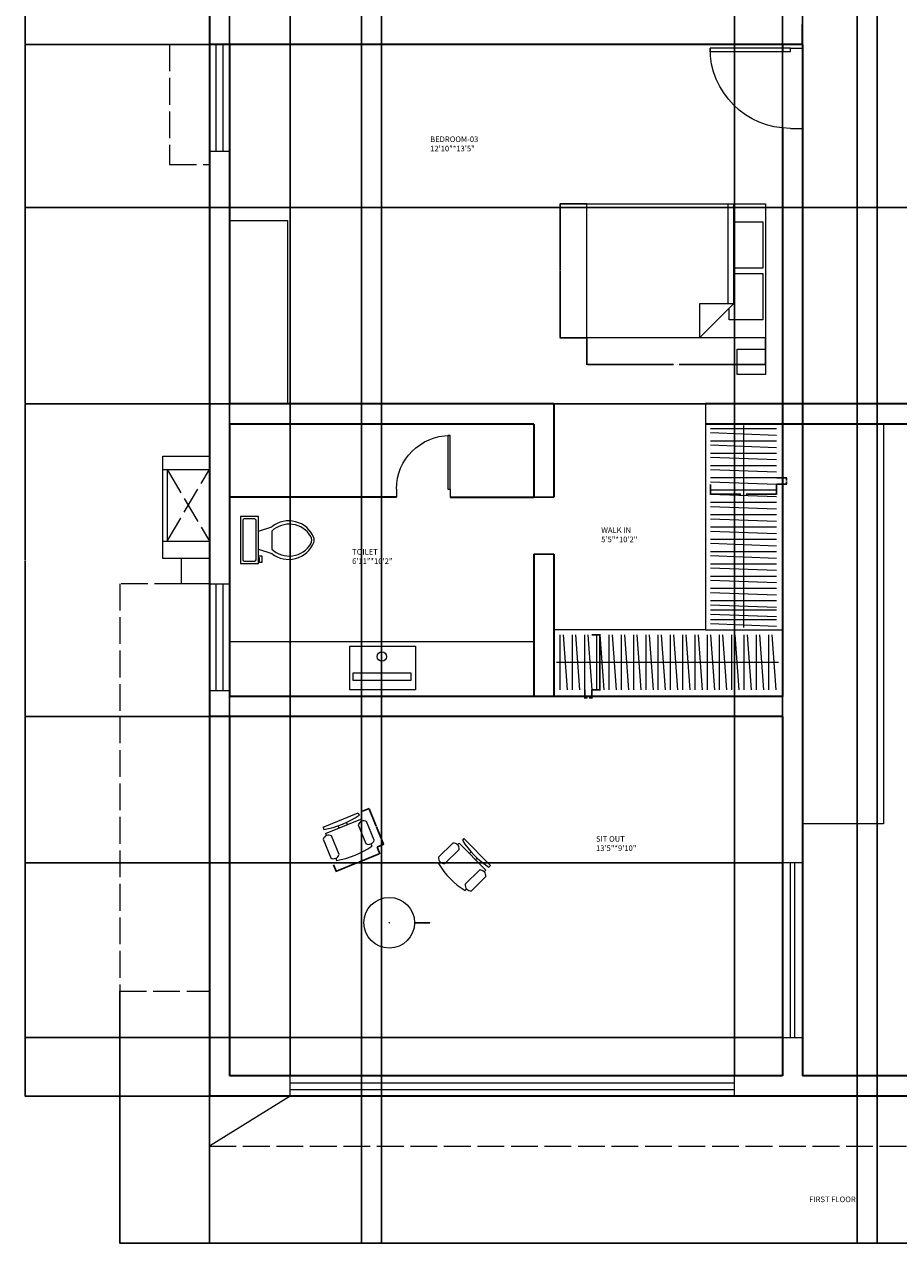
# Model space of a CAD drawing. Units: inches. Extents: x 293720 to 590083, y 155482 to 312405.
# Tile 1 of 4: x 293720 to 294112, y 155482 to 156028. Entities that reach past the tile are written whole.
import ezdxf

# ---------------------------------------------------------------- set-up
doc = ezdxf.new("R2010")
doc.units = ezdxf.units.IN
doc.linetypes.add('ACAD_ISO02W100', pattern=[15, 12, -3])
for name, color, linetype, lineweight in [('A-ANNO-DIMS', 2, 'Continuous', 18), ('A-ANNO-TEXT', 7, 'Continuous', 25), ('A-AREA-IDEN', 7, 'Continuous', 18), ('A-DOOR', 3, 'Continuous', 18), ('A-FLOR-CASE', 8, 'Continuous', 18), ('A-FLOR-FIXT', 9, 'Continuous', 18), ('A-FLOR-OPEN', 8, 'ACAD_ISO02W100', 13), ('A-FLOR-OVHD', 8, 'ACAD_ISO02W100', 13), ('A-FLOR-PROJ', 8, 'Continuous', 18), ('A-FURN', 8, 'Continuous', 18), ('A-GLAZ', 4, 'Continuous', 18), ('A-WALL', 7, 'Continuous', 35), ('A-WALL-HIDN', 7, 'ACAD_ISO02W100', 25)]:
    doc.layers.add(name, color=color, linetype=linetype, lineweight=lineweight)
doc.styles.get("Standard").update_dxf_attribs({"font": 'arial.ttf'})
doc.dimstyles.get("Standard").update_dxf_attribs({"dimtxt": 0.18, "dimasz": 0.18, "dimexe": 0.18, "dimexo": 0.0625, "dimgap": 0.09, "dimtad": 0, "dimtih": 1, "dimtoh": 1, "dimdec": 4, "dimzin": 0, "dimdsep": 46, "dimtxsty": 'Standard', "dimcen": 0.09, "dimadec": 0, "dimazin": 0, "dimtfac": 1, "dimtdec": 4, "dimtofl": 0, "dimtmove": 0, "dimatfit": 3, "dimfxl": 1, "dimtolj": 1, "dimtzin": 0, "dimarcsym": 0})

# ---------------------------------------------------------------- blocks, each defined once
blk = doc.blocks.new('Bed - Queen')
for p, q in [((0, -80.00003), (0, 0)), ((0, 0), (59.99999, 0)), ((59.99999, 0), (59.99999, -80.00003)), ((7.99999, -1.2), (28.79998, -1.2)), ((7.99999, -14.4), (7.99999, -1.2)), ((28.79998, -1.2), (28.79998, -14.4)), ((31.19999, -1.2), (51.99999, -1.2)), ((31.19999, -14.4), (31.19999, -1.2)), ((51.99999, -1.2), (51.99999, -16.4)), ((0, -14.4), (44.8, -14.4)), ((59.99999, -29.6), (44.8, -14.4)), ((44.8, -14.4), (44.8, -29.6)), ((44.8, -16.8), (0, -16.8)), ((51.99999, -16.4), (46.79936, -16.4)), ((44.8, -29.6), (59.99999, -29.6)), ((59.99999, -80.00003), (0, -80.00003))]:
    blk.add_line(p, q)
blk = doc.blocks.new('Toilet - top')
for p, q in [((9.5, -6), (9.5, -2)), ((-10, -8.5), (-8, -8.5)), ((-10, -9.5), (-10, -8.5)), ((-7, -9.5), (-10, -9.5)), ((-8, -8.5), (-8, -8)), ((-7, -8), (-7, -9.5)), ((-4, -8), (-6, -14)), ((4, -8), (6, -14)), ((4, -14), (-4, -14))]:
    blk.add_line(p, q)
blk.add_lwpolyline([(10.5, -8), (10.5, 0), (-10.5, 0), (-10.5, -8)], close=True)
for points in [[(-9.5, -2), (-9.5, -6)], [(8.5, -1), (-8.5, -1)], [(-8.5, -7), (8.5, -7)]]:
    blk.add_lwpolyline(points)
for centre, radius, start, end in [((-8.62, -1.88), 0.884, 81.8699, 188.1301), ((8.62, -1.88), 0.884, 351.8699, 98.1301), ((-8.62, -6.12), 0.884, 171.8699, 278.1301), ((8.62, -6.12), 0.884, 261.8699, 8.1301), ((3.52, -21.58), 12.17, 141.4691, 247.9714), ((4.2, -21.82), 11.33, 136.3677, 238.9468), ((-3.52, -21.58), 12.17, 292.0284, 38.5307), ((-4.2, -21.82), 11.33, 301.053, 43.6321), ((0, -27.88), 4, 245.7318, 294.2682), ((0, -29), 4, 254.8605, 285.1395)]:
    blk.add_arc(centre, radius, start, end)
blk = doc.blocks.new('Chair - Desk')
for p, q in [((-8.5, 0), (-8.5, -1)), ((-8.5, 0), (8.5, 0)), ((8.5, 0), (8.5, -1)), ((-10.5, -5), (-10.5, -14)), ((-8.5, -3), (-8.5, -4)), ((-8.5, -3), (8.5, -3)), ((-6.5, -14), (-6.5, -5)), ((-2, -3), (-2, -1.9355)), ((2, -1.9576), (2, -3)), ((6.5, -5), (6.5, -14)), ((8.5, -3), (8.5, -4)), ((10.5, -14), (10.5, -5)), ((-8.5, -15), (-8.5, -16)), ((8.5, -15), (8.5, -16))]:
    blk.add_line(p, q)
for centre, radius, start, end in [((-8.5, -6.5), 2.5, 36.8699, 143.1301), ((0, 34.625), 36.625, 256.5803, 283.4197), ((8.5, -6.5), 2.5, 36.8699, 143.1301), ((-8.5, -12.5), 2.5, 216.8699, 323.1301), ((0, 19.625), 36.625, 256.5803, 283.4197), ((8.5, -12.5), 2.5, 216.8699, 323.1301)]:
    blk.add_arc(centre, radius, start, end)
blk = doc.blocks.new('*U2')
for p, q in [((0, 0), (0, -6)), ((40, 0), (40, -6))]:
    blk.add_line(p, q)
blk.add_lwpolyline([(0, 0), (0, 40), (1.75, 40), (1.75, 0)], close=True)
blk.add_arc((0, 0), 40, 0, 90)
blk = doc.blocks.new('WIN-48IN')
for p, q in [((0, 9), (48, 9)), ((0, 0), (0, 9)), ((0, 6), (48, 6)), ((48, 9), (48, 0)), ((48, 3), (0, 3)), ((48, 0), (0, 0))]:
    blk.add_line(p, q)
blk = doc.blocks.new('WARDROBE-HANGER-24P54IN')
for p, q in [((0, 0), (0, 24.54)), ((1.33, 24.53), (3.14, 0))]:
    blk.add_line(p, q)
blk = doc.blocks.new('WARDROBE-HANGER-29P64IN')
for p, q in [((0, 2.95), (29.64, 2.95)), ((0, 1.08), (29.64, 0))]:
    blk.add_line(p, q)
blk = doc.blocks.new('*D27')
at = {"layer": 'A-ANNO-DIMS', "color": 0, "lineweight": -2, "transparency": 16777216}
for p, q in [((293974.3, 155754.46), (293978.1, 155754.46)), ((293977.92, 155754.28), (293977.92, 155742.37)), ((293977.92, 155730.1), (293977.92, 155742.01)), ((293974.3, 155729.92), (293978.1, 155729.92))]:
    blk.add_line(p, q, dxfattribs=at)
at = {"layer": 'A-ANNO-DIMS', "color": 0, "lineweight": 100, "transparency": 16777216}
for points in [[(293977.89, 155754.28), (293977.95, 155754.28), (293977.92, 155754.46)], [(293977.89, 155730.1), (293977.95, 155730.1), (293977.92, 155729.92)]]:
    blk.add_solid(points, dxfattribs=at)
at = {"layer": 'Defpoints', "color": 0, "lineweight": 100, "transparency": 16777216}
for p in [(293974.24, 155754.46), (293977.92, 155754.46), (293974.24, 155729.92)]:
    blk.add_point(p, dxfattribs=at)
at = {"layer": 'A-ANNO-DIMS', "color": 0, "transparency": 16777216, "insert": (293977.92, 155742.19), "char_height": 0.18, "attachment_point": 5}
blk.add_mtext('\\A1;HANGER C 25 TYP.', dxfattribs=at)
blk = doc.blocks.new('*D28')
at = {"layer": 'A-ANNO-DIMS', "color": 0, "lineweight": -2, "transparency": 16777216}
for p, q in [((293971.09, 155729.86), (293971.09, 155726.06)), ((293974.24, 155729.86), (293974.24, 155726.06)), ((293971.27, 155726.24), (293972.21, 155726.24)), ((293974.06, 155726.24), (293973.12, 155726.24))]:
    blk.add_line(p, q, dxfattribs=at)
at = {"layer": 'A-ANNO-DIMS', "color": 0, "lineweight": 100, "transparency": 16777216}
for points in [[(293971.27, 155726.27), (293971.27, 155726.21), (293971.09, 155726.24)], [(293974.06, 155726.27), (293974.06, 155726.21), (293974.24, 155726.24)]]:
    blk.add_solid(points, dxfattribs=at)
at = {"layer": 'Defpoints', "color": 0, "lineweight": 100, "transparency": 16777216}
for p in [(293971.09, 155729.92), (293974.24, 155729.92), (293974.24, 155726.24)]:
    blk.add_point(p, dxfattribs=at)
at = {"layer": 'A-ANNO-DIMS', "color": 0, "transparency": 16777216, "insert": (293972.66, 155726.24), "char_height": 0.18, "attachment_point": 5}
blk.add_mtext('\\A1;3 TYP.', dxfattribs=at)
blk = doc.blocks.new('*D29')
at = {"layer": 'A-ANNO-DIMS', "color": 0, "lineweight": -2, "transparency": 16777216}
for p, q in [((294027.35, 155821.9), (294027.35, 155817.34)), ((294027.53, 155817.52), (294040.95, 155817.52)), ((294056.82, 155817.52), (294043.4, 155817.52)), ((294057, 155821.9), (294057, 155817.34))]:
    blk.add_line(p, q, dxfattribs=at)
at = {"layer": 'A-ANNO-DIMS', "color": 0, "lineweight": 100, "transparency": 16777216}
for points in [[(294027.53, 155817.55), (294027.53, 155817.49), (294027.35, 155817.52)], [(294056.82, 155817.55), (294056.82, 155817.49), (294057, 155817.52)]]:
    blk.add_solid(points, dxfattribs=at)
at = {"layer": 'Defpoints', "color": 0, "lineweight": 100, "transparency": 16777216}
for p in [(294027.35, 155821.96), (294057, 155821.96), (294057, 155817.52)]:
    blk.add_point(p, dxfattribs=at)
at = {"layer": 'A-ANNO-DIMS', "color": 0, "transparency": 16777216, "insert": (294042.18, 155817.52), "char_height": 0.18, "attachment_point": 5}
blk.add_mtext('\\A1;HANGER D 30 TYP.', dxfattribs=at)
blk = doc.blocks.new('*D30')
at = {"layer": 'A-ANNO-DIMS', "color": 0, "lineweight": -2, "transparency": 16777216}
for p, q in [((294057.06, 155824.91), (294061.63, 155824.91)), ((294061.45, 155824.73), (294061.45, 155823.62)), ((294061.45, 155822.14), (294061.45, 155823.26)), ((294057.06, 155821.96), (294061.63, 155821.96))]:
    blk.add_line(p, q, dxfattribs=at)
at = {"layer": 'A-ANNO-DIMS', "color": 0, "lineweight": 100, "transparency": 16777216}
for points in [[(294061.42, 155824.73), (294061.48, 155824.73), (294061.45, 155824.91)], [(294061.42, 155822.14), (294061.48, 155822.14), (294061.45, 155821.96)]]:
    blk.add_solid(points, dxfattribs=at)
at = {"layer": 'Defpoints', "color": 0, "lineweight": 100, "transparency": 16777216}
for p in [(294057, 155824.91), (294061.45, 155824.91), (294057, 155821.96)]:
    blk.add_point(p, dxfattribs=at)
at = {"layer": 'A-ANNO-DIMS', "color": 0, "transparency": 16777216, "insert": (294061.45, 155823.44), "char_height": 0.18, "attachment_point": 5}
blk.add_mtext('\\A1;3 TYP.', dxfattribs=at)
blk = doc.blocks.new('*D41')
at = {"layer": 'A-ANNO-DIMS', "color": 0, "lineweight": -2, "transparency": 16777216}
for p, q in [((293878.12, 155659.4), (293879.36, 155656.38)), ((293879.13, 155656.48), (293870.02, 155652.76)), ((293858.69, 155651.46), (293859.92, 155648.43)), ((293860.02, 155648.67), (293869.13, 155652.39))]:
    blk.add_line(p, q, dxfattribs=at)
at = {"layer": 'A-ANNO-DIMS', "color": 0, "lineweight": 100, "transparency": 16777216}
for points in [[(293879.12, 155656.51), (293879.14, 155656.45), (293879.29, 155656.55)], [(293860.01, 155648.69), (293860.03, 155648.64), (293859.85, 155648.6)]]:
    blk.add_solid(points, dxfattribs=at)
at = {"layer": 'Defpoints', "color": 0, "lineweight": 100, "transparency": 16777216}
for p in [(293878.1, 155659.46), (293879.29, 155656.55), (293858.66, 155651.51)]:
    blk.add_point(p, dxfattribs=at)
at = {"layer": 'A-ANNO-DIMS', "color": 0, "transparency": 16777216, "insert": (293869.57, 155652.57), "char_height": 0.18, "attachment_point": 5}
blk.add_mtext('\\A1;CHAIR 21 TYP.', dxfattribs=at)
blk = doc.blocks.new('*D42')
at = {"layer": 'A-ANNO-DIMS', "color": 0, "lineweight": -2, "transparency": 16777216}
for p, q in [((293871.6, 155675.53), (293874.62, 155676.77)), ((293874.53, 155676.53), (293877.66, 155668.86)), ((293880.95, 155660.82), (293877.81, 155668.49)), ((293878.16, 155659.48), (293881.18, 155660.72))]:
    blk.add_line(p, q, dxfattribs=at)
at = {"layer": 'A-ANNO-DIMS', "color": 0, "lineweight": 100, "transparency": 16777216}
for points in [[(293874.55, 155676.54), (293874.5, 155676.52), (293874.46, 155676.7)], [(293880.98, 155660.83), (293880.92, 155660.81), (293881.02, 155660.65)]]:
    blk.add_solid(points, dxfattribs=at)
at = {"layer": 'Defpoints', "color": 0, "lineweight": 100, "transparency": 16777216}
for p in [(293871.54, 155675.51), (293874.46, 155676.7), (293878.1, 155659.46)]:
    blk.add_point(p, dxfattribs=at)
at = {"layer": 'A-ANNO-DIMS', "color": 0, "transparency": 16777216, "insert": (293877.74, 155668.68), "char_height": 0.18, "attachment_point": 5}
blk.add_mtext('\\A1;17 TYP.', dxfattribs=at)
blk = doc.blocks.new('*D43')
at = {"layer": 'A-ANNO-DIMS', "color": 0, "lineweight": -2, "transparency": 16777216}
for p, q in [((293972.1, 155887.5), (293972.1, 155875.38)), ((294052.1, 155887.5), (294052.1, 155875.38)), ((293972.28, 155875.56), (294010.8, 155875.56)), ((294051.92, 155875.56), (294013.4, 155875.56))]:
    blk.add_line(p, q, dxfattribs=at)
at = {"layer": 'A-ANNO-DIMS', "color": 0, "lineweight": 100, "transparency": 16777216}
for points in [[(293972.28, 155875.59), (293972.28, 155875.53), (293972.1, 155875.56)], [(294051.92, 155875.59), (294051.92, 155875.53), (294052.1, 155875.56)]]:
    blk.add_solid(points, dxfattribs=at)
at = {"layer": 'Defpoints', "color": 0, "lineweight": 100, "transparency": 16777216}
for p in [(293972.1, 155887.56), (294052.1, 155887.56), (294052.1, 155875.56)]:
    blk.add_point(p, dxfattribs=at)
at = {"layer": 'A-ANNO-DIMS', "color": 0, "transparency": 16777216, "insert": (294012.1, 155875.56), "char_height": 0.18, "attachment_point": 5}
blk.add_mtext('\\A1;QUEEN BED 80 TYP.', dxfattribs=at)
blk = doc.blocks.new('*D44')
at = {"layer": 'A-ANNO-DIMS', "color": 0, "lineweight": -2, "transparency": 16777216}
for p, q in [((293972.04, 155947.56), (293959.92, 155947.56)), ((293960.1, 155947.38), (293960.1, 155917.74)), ((293960.1, 155887.74), (293960.1, 155917.38)), ((293972.04, 155887.56), (293959.92, 155887.56))]:
    blk.add_line(p, q, dxfattribs=at)
at = {"layer": 'A-ANNO-DIMS', "color": 0, "lineweight": 100, "transparency": 16777216}
for points in [[(293960.07, 155947.38), (293960.13, 155947.38), (293960.1, 155947.56)], [(293960.07, 155887.74), (293960.13, 155887.74), (293960.1, 155887.56)]]:
    blk.add_solid(points, dxfattribs=at)
at = {"layer": 'Defpoints', "color": 0, "lineweight": 100, "transparency": 16777216}
for p in [(293972.1, 155947.56), (293960.1, 155887.56), (293972.1, 155887.56)]:
    blk.add_point(p, dxfattribs=at)
at = {"layer": 'A-ANNO-DIMS', "color": 0, "transparency": 16777216, "insert": (293960.1, 155917.56), "char_height": 0.18, "attachment_point": 5}
blk.add_mtext('\\A1;60 TYP.', dxfattribs=at)
blk = doc.blocks.new('*D53')
at = {"layer": 'A-ANNO-DIMS', "color": 0, "lineweight": -2, "transparency": 16777216}
for p, q in [((294499.07, 156062.55), (294499.07, 155481.85)), ((293762.89, 155594.88), (293762.89, 155481.85)), ((293763.07, 155482.03), (294130.59, 155482.03)), ((294498.89, 155482.03), (294131.37, 155482.03))]:
    blk.add_line(p, q, dxfattribs=at)
at = {"layer": 'A-ANNO-DIMS', "color": 0, "lineweight": 100, "transparency": 16777216}
for points in [[(293763.07, 155482.06), (293763.07, 155482), (293762.89, 155482.03)], [(294498.89, 155482.06), (294498.89, 155482), (294499.07, 155482.03)]]:
    blk.add_solid(points, dxfattribs=at)
at = {"layer": 'Defpoints', "color": 0, "lineweight": 100, "transparency": 16777216}
for p in [(294499.07, 156062.61), (293762.89, 155594.94), (294499.07, 155482.03)]:
    blk.add_point(p, dxfattribs=at)
at = {"layer": 'A-ANNO-DIMS', "color": 0, "transparency": 16777216, "insert": (294130.98, 155482.03), "char_height": 0.18, "attachment_point": 5}
blk.add_mtext('\\A1;736.2', dxfattribs=at)
blk = doc.blocks.new('*D56')
at = {"layer": 'A-ANNO-DIMS', "color": 0, "lineweight": -2, "transparency": 16777216}
for p, q in [((293803.09, 156304.87), (293803.09, 155481.85)), ((293871.09, 156304.87), (293871.09, 155481.85)), ((293803.27, 155482.03), (293836.87, 155482.03)), ((293870.91, 155482.03), (293837.31, 155482.03))]:
    blk.add_line(p, q, dxfattribs=at)
at = {"layer": 'A-ANNO-DIMS', "color": 0, "lineweight": 100, "transparency": 16777216}
for points in [[(293803.27, 155482.06), (293803.27, 155482), (293803.09, 155482.03)], [(293870.91, 155482.06), (293870.91, 155482), (293871.09, 155482.03)]]:
    blk.add_solid(points, dxfattribs=at)
at = {"layer": 'Defpoints', "color": 0, "lineweight": 100, "transparency": 16777216}
for p in [(293803.09, 156304.93), (293871.09, 156304.93), (293871.09, 155482.03)]:
    blk.add_point(p, dxfattribs=at)
at = {"layer": 'A-ANNO-DIMS', "color": 0, "transparency": 16777216, "insert": (293837.09, 155482.03), "char_height": 0.18, "attachment_point": 5}
blk.add_mtext('\\A1;68', dxfattribs=at)
blk = doc.blocks.new('*D57')
at = {"layer": 'A-ANNO-DIMS', "color": 0, "lineweight": -2, "transparency": 16777216}
for p, q in [((293880.093104, 156304.865707), (293880.093104, 155481.8534)), ((294093.093104, 156304.865707), (294093.093104, 155481.8534)), ((293880.273104, 155482.0334), (293986.302722, 155482.0334)), ((294092.913104, 155482.0334), (293986.883486, 155482.0334))]:
    blk.add_line(p, q, dxfattribs=at)
at = {"layer": 'A-ANNO-DIMS', "color": 0, "lineweight": 100, "transparency": 16777216}
for points in [[(293880.273104, 155482.0634), (293880.273104, 155482.0034), (293880.093104, 155482.0334)], [(294092.913104, 155482.0634), (294092.913104, 155482.0034), (294093.093104, 155482.0334)]]:
    blk.add_solid(points, dxfattribs=at)
at = {"layer": 'Defpoints', "color": 0, "lineweight": 100, "transparency": 16777216}
for p in [(293880.093104, 156304.928207), (294093.093104, 156304.928207), (294093.093104, 155482.0334)]:
    blk.add_point(p, dxfattribs=at)
at = {"layer": 'A-ANNO-DIMS', "color": 0, "transparency": 16777216, "insert": (293986.593104, 155482.0334), "char_height": 0.18, "attachment_point": 5}
blk.add_mtext('\\A1;213', dxfattribs=at)
blk = doc.blocks.new('*D58')
at = {"layer": 'A-ANNO-DIMS', "color": 0, "lineweight": -2, "transparency": 16777216}
for p, q in [((294102.09, 156200.87), (294102.09, 155481.85)), ((294173.09, 156200.87), (294173.09, 155481.85)), ((294102.27, 155482.03), (294137.39, 155482.03)), ((294172.91, 155482.03), (294137.79, 155482.03))]:
    blk.add_line(p, q, dxfattribs=at)
at = {"layer": 'A-ANNO-DIMS', "color": 0, "lineweight": 100, "transparency": 16777216}
for points in [[(294102.27, 155482.06), (294102.27, 155482), (294102.09, 155482.03)], [(294172.91, 155482.06), (294172.91, 155482), (294173.09, 155482.03)]]:
    blk.add_solid(points, dxfattribs=at)
at = {"layer": 'Defpoints', "color": 0, "lineweight": 100, "transparency": 16777216}
for p in [(294102.09, 156200.93), (294173.09, 156200.93), (294173.09, 155482.03)]:
    blk.add_point(p, dxfattribs=at)
at = {"layer": 'A-ANNO-DIMS', "color": 0, "transparency": 16777216, "insert": (294137.59, 155482.03), "char_height": 0.18, "attachment_point": 5}
blk.add_mtext('\\A1;71', dxfattribs=at)
blk = doc.blocks.new('*D61')
at = {"layer": 'A-ANNO-DIMS', "color": 0, "lineweight": -2, "transparency": 16777216}
for p, q in [((293803.03, 155717.93), (293720.36, 155717.93)), ((293720.54, 155717.75), (293720.54, 155633.11)), ((293720.54, 155548.11), (293720.54, 155632.75)), ((293803.03, 155547.93), (293720.36, 155547.93))]:
    blk.add_line(p, q, dxfattribs=at)
at = {"layer": 'A-ANNO-DIMS', "color": 0, "lineweight": 100, "transparency": 16777216}
for points in [[(293720.51, 155717.75), (293720.57, 155717.75), (293720.54, 155717.93)], [(293720.51, 155548.11), (293720.57, 155548.11), (293720.54, 155547.93)]]:
    blk.add_solid(points, dxfattribs=at)
at = {"layer": 'Defpoints', "color": 0, "lineweight": 100, "transparency": 16777216}
for p in [(293720.54, 155717.93), (293803.09, 155717.93), (293803.09, 155547.93)]:
    blk.add_point(p, dxfattribs=at)
at = {"layer": 'A-ANNO-DIMS', "color": 0, "transparency": 16777216, "insert": (293720.54, 155632.93), "char_height": 0.18, "attachment_point": 5}
blk.add_mtext('\\A1;170', dxfattribs=at)
blk = doc.blocks.new('*D62')
at = {"layer": 'A-ANNO-DIMS', "color": 0, "lineweight": -2, "transparency": 16777216}
for p, q in [((293812.03, 155857.93), (293720.36, 155857.93)), ((293720.54, 155857.75), (293720.54, 155788.11)), ((293720.54, 155718.11), (293720.54, 155787.75)), ((293803.03, 155717.93), (293720.36, 155717.93))]:
    blk.add_line(p, q, dxfattribs=at)
at = {"layer": 'A-ANNO-DIMS', "color": 0, "lineweight": 100, "transparency": 16777216}
for points in [[(293720.51, 155857.75), (293720.57, 155857.75), (293720.54, 155857.93)], [(293720.51, 155718.11), (293720.57, 155718.11), (293720.54, 155717.93)]]:
    blk.add_solid(points, dxfattribs=at)
at = {"layer": 'Defpoints', "color": 0, "lineweight": 100, "transparency": 16777216}
for p in [(293720.54, 155857.93), (293812.09, 155857.93), (293803.09, 155717.93)]:
    blk.add_point(p, dxfattribs=at)
at = {"layer": 'A-ANNO-DIMS', "color": 0, "transparency": 16777216, "insert": (293720.54, 155787.93), "char_height": 0.18, "attachment_point": 5}
blk.add_mtext('\\A1;140', dxfattribs=at)
blk = doc.blocks.new('*D63')
at = {"layer": 'A-ANNO-DIMS', "color": 0, "lineweight": -2, "transparency": 16777216}
for p, q in [((293812.03, 156018.93), (293720.36, 156018.93)), ((293720.54, 156018.75), (293720.54, 155938.61)), ((293720.54, 155858.11), (293720.54, 155938.25)), ((293812.03, 155857.93), (293720.36, 155857.93))]:
    blk.add_line(p, q, dxfattribs=at)
at = {"layer": 'A-ANNO-DIMS', "color": 0, "lineweight": 100, "transparency": 16777216}
for points in [[(293720.51, 156018.75), (293720.57, 156018.75), (293720.54, 156018.93)], [(293720.51, 155858.11), (293720.57, 155858.11), (293720.54, 155857.93)]]:
    blk.add_solid(points, dxfattribs=at)
at = {"layer": 'Defpoints', "color": 0, "lineweight": 100, "transparency": 16777216}
for p in [(293720.54, 156018.93), (293812.09, 156018.93), (293812.09, 155857.93)]:
    blk.add_point(p, dxfattribs=at)
at = {"layer": 'A-ANNO-DIMS', "color": 0, "transparency": 16777216, "insert": (293720.54, 155938.43), "char_height": 0.18, "attachment_point": 5}
blk.add_mtext('\\A1;161', dxfattribs=at)
blk = doc.blocks.new('*D64')
at = {"layer": 'A-ANNO-DIMS', "color": 0, "lineweight": -2, "transparency": 16777216}
for p, q in [((293803.03, 156166.43), (293720.36, 156166.43)), ((293720.54, 156166.25), (293720.54, 156092.86)), ((293720.54, 156019.11), (293720.54, 156092.5)), ((293812.03, 156018.93), (293720.36, 156018.93))]:
    blk.add_line(p, q, dxfattribs=at)
at = {"layer": 'A-ANNO-DIMS', "color": 0, "lineweight": 100, "transparency": 16777216}
for points in [[(293720.51, 156166.25), (293720.57, 156166.25), (293720.54, 156166.43)], [(293720.51, 156019.11), (293720.57, 156019.11), (293720.54, 156018.93)]]:
    blk.add_solid(points, dxfattribs=at)
at = {"layer": 'Defpoints', "color": 0, "lineweight": 100, "transparency": 16777216}
for p in [(293720.54, 156166.43), (293803.09, 156166.43), (293812.09, 156018.93)]:
    blk.add_point(p, dxfattribs=at)
at = {"layer": 'A-ANNO-DIMS', "color": 0, "transparency": 16777216, "insert": (293720.54, 156092.68), "char_height": 0.18, "attachment_point": 5}
blk.add_mtext('\\A1;147.5', dxfattribs=at)
blk = doc.blocks.new('*D66')
at = {"layer": 'A-ANNO-DIMS', "color": 0, "lineweight": -2, "transparency": 16777216}
for p, q in [((293812.09, 155556.99), (293812.09, 156377.57)), ((293812.27, 156377.39), (293825.26, 156377.39)), ((293839.03, 156377.39), (293826.05, 156377.39)), ((293839.21, 155556.99), (293839.21, 156377.57))]:
    blk.add_line(p, q, dxfattribs=at)
at = {"layer": 'A-ANNO-DIMS', "color": 0, "lineweight": 100, "transparency": 16777216}
for points in [[(293812.27, 156377.42), (293812.27, 156377.36), (293812.09, 156377.39)], [(293839.03, 156377.42), (293839.03, 156377.36), (293839.21, 156377.39)]]:
    blk.add_solid(points, dxfattribs=at)
at = {"layer": 'Defpoints', "color": 0, "lineweight": 100, "transparency": 16777216}
for p in [(293839.21, 156377.39), (293812.09, 155556.93), (293839.21, 155556.93)]:
    blk.add_point(p, dxfattribs=at)
at = {"layer": 'A-ANNO-DIMS', "color": 0, "transparency": 16777216, "insert": (293825.65, 156377.39), "char_height": 0.18, "attachment_point": 5}
blk.add_mtext('\\A1;27.12', dxfattribs=at)
blk = doc.blocks.new('*D67')
at = {"layer": 'A-ANNO-DIMS', "color": 0, "lineweight": -2, "transparency": 16777216}
for p, q in [((293839.21, 155556.99), (293839.21, 156377.57)), ((293839.39, 156377.39), (293938.24, 156377.39)), ((294038, 156377.39), (293939.15, 156377.39)), ((294038.18, 155556.99), (294038.18, 156377.57))]:
    blk.add_line(p, q, dxfattribs=at)
at = {"layer": 'A-ANNO-DIMS', "color": 0, "lineweight": 100, "transparency": 16777216}
for points in [[(293839.39, 156377.42), (293839.39, 156377.36), (293839.21, 156377.39)], [(294038, 156377.42), (294038, 156377.36), (294038.18, 156377.39)]]:
    blk.add_solid(points, dxfattribs=at)
at = {"layer": 'Defpoints', "color": 0, "lineweight": 100, "transparency": 16777216}
for p in [(294038.18, 156377.39), (293839.21, 155556.93), (294038.18, 155556.93)]:
    blk.add_point(p, dxfattribs=at)
at = {"layer": 'A-ANNO-DIMS', "color": 0, "transparency": 16777216, "insert": (293938.7, 156377.39), "char_height": 0.18, "attachment_point": 5}
blk.add_mtext('\\A1;198.97', dxfattribs=at)
blk = doc.blocks.new('*D68')
at = {"layer": 'A-ANNO-DIMS', "color": 0, "lineweight": -2, "transparency": 16777216}
for p, q in [((294038.180795, 155556.990707), (294038.180795, 156377.567612)), ((294038.360795, 156377.387612), (294048.417601, 156377.387612)), ((294059.406085, 156377.387612), (294049.349279, 156377.387612)), ((294059.586085, 155556.990707), (294059.586085, 156377.567612))]:
    blk.add_line(p, q, dxfattribs=at)
at = {"layer": 'A-ANNO-DIMS', "color": 0, "lineweight": 100, "transparency": 16777216}
for points in [[(294038.360795, 156377.417612), (294038.360795, 156377.357612), (294038.180795, 156377.387612)], [(294059.406085, 156377.417612), (294059.406085, 156377.357612), (294059.586085, 156377.387612)]]:
    blk.add_solid(points, dxfattribs=at)
at = {"layer": 'Defpoints', "color": 0, "lineweight": 100, "transparency": 16777216}
for p in [(294059.586085, 156377.387612), (294038.180795, 155556.928207), (294059.586085, 155556.928207)]:
    blk.add_point(p, dxfattribs=at)
at = {"layer": 'A-ANNO-DIMS', "color": 0, "transparency": 16777216, "insert": (294048.88344, 156377.387612), "char_height": 0.18, "attachment_point": 5}
blk.add_mtext('\\A1;21.405', dxfattribs=at)
blk = doc.blocks.new('*D69')
at = {"layer": 'A-ANNO-DIMS', "color": 0, "lineweight": -2, "transparency": 16777216}
for p, q in [((294068.586085, 155556.990707), (294068.586085, 156377.567612)), ((294068.766085, 156377.387612), (294096.611145, 156377.387612)), ((294125.103763, 156377.387612), (294097.258703, 156377.387612)), ((294125.283763, 155556.990707), (294125.283763, 156377.567612))]:
    blk.add_line(p, q, dxfattribs=at)
at = {"layer": 'A-ANNO-DIMS', "color": 0, "lineweight": 100, "transparency": 16777216}
for points in [[(294068.766085, 156377.417612), (294068.766085, 156377.357612), (294068.586085, 156377.387612)], [(294125.103763, 156377.417612), (294125.103763, 156377.357612), (294125.283763, 156377.387612)]]:
    blk.add_solid(points, dxfattribs=at)
at = {"layer": 'Defpoints', "color": 0, "lineweight": 100, "transparency": 16777216}
for p in [(294125.283763, 156377.387612), (294068.586085, 155556.928207), (294125.283763, 155556.928207)]:
    blk.add_point(p, dxfattribs=at)
at = {"layer": 'A-ANNO-DIMS', "color": 0, "transparency": 16777216, "insert": (294096.934924, 156377.387612), "char_height": 0.18, "attachment_point": 5}
blk.add_mtext('\\A1;56.7', dxfattribs=at)
blk = doc.blocks.new('*D72')
at = {"layer": 'A-ANNO-DIMS', "color": 0, "lineweight": -2, "transparency": 16777216}
for p, q in [((294321.18, 155945.93), (293720.36, 155945.93)), ((293720.54, 155945.75), (293720.54, 155902.11)), ((293720.54, 155858.11), (293720.54, 155901.75)), ((294321.18, 155857.93), (293720.36, 155857.93))]:
    blk.add_line(p, q, dxfattribs=at)
at = {"layer": 'A-ANNO-DIMS', "color": 0, "lineweight": 100, "transparency": 16777216}
for points in [[(293720.51, 155945.75), (293720.57, 155945.75), (293720.54, 155945.93)], [(293720.51, 155858.11), (293720.57, 155858.11), (293720.54, 155857.93)]]:
    blk.add_solid(points, dxfattribs=at)
at = {"layer": 'Defpoints', "color": 0, "lineweight": 100, "transparency": 16777216}
for p in [(293720.54, 155945.93), (294321.24, 155945.93), (294321.24, 155857.93)]:
    blk.add_point(p, dxfattribs=at)
at = {"layer": 'A-ANNO-DIMS', "color": 0, "transparency": 16777216, "insert": (293720.54, 155901.93), "char_height": 0.18, "attachment_point": 5}
blk.add_mtext('\\A1;88', dxfattribs=at)
blk = doc.blocks.new('*D75')
at = {"layer": 'A-ANNO-DIMS', "color": 0, "lineweight": -2, "transparency": 16777216}
for p, q in [((294059.52, 155652.4), (293720.36, 155652.4)), ((293720.54, 155652.22), (293720.54, 155613.45)), ((293720.54, 155574.32), (293720.54, 155613.09)), ((294059.52, 155574.14), (293720.36, 155574.14))]:
    blk.add_line(p, q, dxfattribs=at)
at = {"layer": 'A-ANNO-DIMS', "color": 0, "lineweight": 100, "transparency": 16777216}
for points in [[(293720.51, 155652.22), (293720.57, 155652.22), (293720.54, 155652.4)], [(293720.51, 155574.32), (293720.57, 155574.32), (293720.54, 155574.14)]]:
    blk.add_solid(points, dxfattribs=at)
at = {"layer": 'Defpoints', "color": 0, "lineweight": 100, "transparency": 16777216}
for p in [(293720.54, 155652.4), (294059.59, 155652.4), (294059.59, 155574.14)]:
    blk.add_point(p, dxfattribs=at)
at = {"layer": 'A-ANNO-DIMS', "color": 0, "transparency": 16777216, "insert": (293720.54, 155613.27), "char_height": 0.18, "attachment_point": 5}
blk.add_mtext('\\A1;78.26', dxfattribs=at)
blk = doc.blocks.new('*D78')
at = {"layer": 'A-ANNO-DIMS', "color": 0, "lineweight": -2, "transparency": 16777216}
for p, q in [((293883.49, 155625.56), (293883.67, 155625.56)), ((293883.58, 155625.47), (293883.58, 155625.65)), ((293901.74, 155625.56), (293895.11, 155625.56))]:
    blk.add_line(p, q, dxfattribs=at)
at = {"layer": 'A-ANNO-DIMS', "color": 0, "lineweight": 100, "transparency": 16777216}
blk.add_solid([(293895.11, 155625.59), (293895.11, 155625.53), (293894.93, 155625.56)], dxfattribs=at)
at = {"layer": 'Defpoints', "color": 0, "lineweight": 100, "transparency": 16777216}
for p in [(293872.24, 155625.56), (293894.93, 155625.56)]:
    blk.add_point(p, dxfattribs=at)
at = {"layer": 'A-ANNO-DIMS', "color": 0, "transparency": 16777216, "insert": (293902.3, 155625.56), "char_height": 0.18, "attachment_point": 5}
blk.add_mtext('\\A1;∅22.692', dxfattribs=at)

msp = doc.modelspace()

# ---------------------------------------------------------------- linework, layer by layer
at = {"layer": 'A-FLOR-CASE'}
for p, q in [((293812.0931, 155940.1253), (293837.9841, 155940.1253)), ((293837.9841, 155940.1253), (293837.9841, 155857.9282)), ((294025.2305, 155857.9282), (294025.2305, 155756.6999)), ((294042.2003, 155848.2167), (294042.2003, 155764.4281)), ((294104.856, 155848.9282), (294104.856, 155669.844)), ((294042.2003, 155764.4281), (294042.2003, 155757.8352)), ((293812.0931, 155751.5862), (293948.3101, 155751.5862)), ((294025.2305, 155756.6999), (293957.3101, 155756.6999)), ((294025.2305, 155756.6999), (294059.5861, 155756.6999)), ((293958.4339, 155742.2401), (294057.8148, 155742.2401)), ((294104.856, 155669.844), (294068.5861, 155669.844))]:
    msp.add_line(p, q, dxfattribs=at)
at = {"layer": 'A-FLOR-FIXT'}
for p, q in [((293867.4587, 155737.5237), (293893.1801, 155737.5237)), ((293867.4587, 155734.0238), (293867.4587, 155737.5237)), ((293893.1801, 155737.5237), (293893.1801, 155734.0238)), ((293893.1801, 155734.0238), (293867.4587, 155734.0238))]:
    msp.add_line(p, q, dxfattribs=at)
msp.add_lwpolyline([(293865.9092, 155749.3986), (293895.3459, 155749.3986), (293895.3459, 155729.8631), (293865.9092, 155729.8631)], close=True, dxfattribs=at)
msp.add_circle((293880.2971, 155744.78), 2.1189, dxfattribs=at)
at = {"layer": 'A-FLOR-OPEN'}
for p, q in [((293784.2178, 155796.4872), (293803.0931, 155828.5172)), ((293784.2178, 155828.5172), (293803.0931, 155796.4872))]:
    msp.add_line(p, q, dxfattribs=at)
at = {"layer": 'A-FLOR-OVHD'}
for p, q in [((293803.0931, 156018.9282), (293785.2239, 156018.9282)), ((293785.2239, 156018.9282), (293785.2239, 155965.1062)), ((293785.2239, 155965.1062), (293803.0931, 155965.1062)), ((293790.4983, 155777.4328), (293762.8891, 155777.4328)), ((293762.8891, 155777.4328), (293762.8891, 155717.9282)), ((293803.0931, 155717.9282), (293762.8891, 155717.9282)), ((293762.8891, 155717.9282), (293762.8891, 155594.9386)), ((293762.8891, 155594.9386), (293803.0931, 155594.9386)), ((293803.0931, 155525.5662), (294266.2589, 155525.5662))]:
    msp.add_line(p, q, dxfattribs=at)
at = {"layer": 'A-FLOR-PROJ'}
for p, q in [((293782.1825, 155828.5172), (293782.1825, 155834.5389)), ((293782.1825, 155834.5389), (293803.0931, 155834.5389)), ((293782.1825, 155796.4872), (293782.1825, 155828.5172)), ((293782.1825, 155828.5172), (293803.0931, 155828.5172)), ((293784.2178, 155828.5172), (293784.2178, 155796.4872)), ((293782.1825, 155788.7451), (293782.1825, 155796.4872)), ((293782.1825, 155796.4872), (293803.0931, 155796.4872)), ((293803.0931, 155788.7451), (293782.1825, 155788.7451)), ((293790.4983, 155777.4328), (293790.4983, 155788.7451)), ((293803.0931, 155777.4328), (293790.4983, 155777.4328)), ((293839.2106, 155547.9282), (293803.0931, 155525.5662)), ((293803.0931, 155525.5662), (293803.0931, 155547.9282))]:
    msp.add_line(p, q, dxfattribs=at)
at = {"layer": 'A-FURN'}
msp.add_lwpolyline([(294039.2942, 155882.4281), (294052.0946, 155882.4281), (294052.0946, 155871.0591), (294039.2942, 155871.0591)], close=True, dxfattribs=at)
msp.add_circle((293883.5815, 155625.5625), 11.3462, dxfattribs=at)
at = {"layer": 'A-GLAZ'}
for p, q in [((294068.5861, 155652.3986), (294059.5861, 155652.3986)), ((294063.0468, 155652.3537), (294063.0468, 155574.1424)), ((294064.9463, 155652.3986), (294064.9463, 155574.1424)), ((294059.5861, 155574.1424), (294068.5861, 155574.1424)), ((293839.2106, 155547.9282), (293839.2106, 155556.9282)), ((294038.1808, 155547.9282), (294038.1808, 155556.9282)), ((293839.2106, 155553.9282), (294038.1808, 155553.9282)), ((293839.2106, 155550.9282), (294038.1808, 155550.9282))]:
    msp.add_line(p, q, dxfattribs=at)
at = {"layer": 'A-WALL'}
for p, q in [((293803.0931, 156313.9282), (293803.0931, 155547.9282)), ((294068.5861, 156018.9282), (294068.5861, 156027.9282)), ((294068.5861, 156018.9282), (293803.0931, 156018.9282)), ((293812.0931, 156018.9282), (293812.0931, 155857.9282)), ((294059.5861, 156018.9282), (294059.5861, 156015.7616)), ((294068.5861, 156018.9282), (294068.5861, 155556.9282)), ((294059.5861, 155981.517), (294059.5861, 155726.9282)), ((293957.3101, 155857.9282), (293812.0931, 155857.9282)), ((293957.3101, 155857.9282), (293957.3101, 155816.1828)), ((294463.2763, 155857.9282), (294025.2305, 155857.9282)), ((293812.0931, 155848.9282), (293812.0931, 155726.9282)), ((293948.3101, 155848.9282), (293812.0931, 155848.9282)), ((293948.3101, 155848.9282), (293948.3101, 155816.1828)), ((294144.2603, 155848.9282), (294025.2305, 155848.9282)), ((293886.7893, 155816.1828), (293812.0931, 155816.1828)), ((293910.7893, 155816.1828), (293948.3101, 155816.1828)), ((293948.3101, 155790.5985), (293948.3101, 155726.9282)), ((293957.3101, 155790.5985), (293957.3101, 155726.9282)), ((294059.5861, 155726.9282), (293812.0931, 155726.9282)), ((294059.5861, 155717.9282), (293803.0931, 155717.9282)), ((293812.0931, 155717.9282), (293812.0931, 155556.9282)), ((294059.5861, 155717.9282), (294059.5861, 155556.9282)), ((294059.5861, 155556.9282), (293812.0931, 155556.9282)), ((294245.5861, 155556.9282), (294068.5861, 155556.9282)), ((294274.4362, 155547.9282), (293803.0931, 155547.9282))]:
    msp.add_line(p, q, dxfattribs=at)
at = {"layer": 'A-WALL-HIDN'}
for p, q in [((293948.3101, 155816.1828), (293957.3101, 155816.1828)), ((293948.3101, 155790.5985), (293957.3101, 155790.5985))]:
    msp.add_line(p, q, dxfattribs=at)

# ---------------------------------------------------------------- block references
at = {"layer": 'A-DOOR', "xscale": -0.9, "yscale": 0.9, "zscale": 0.9, "rotation": 90}
msp.add_blockref('*U2', (294063.1861, 156017.3366), dxfattribs=at)
at = {"layer": 'A-DOOR', "xscale": -0.6, "yscale": 0.6, "zscale": 0.6}
msp.add_blockref('*U2', (293910.7893, 155819.7828), dxfattribs=at)
at = {"layer": 'A-FLOR-CASE'}
for name, p in [('WARDROBE-HANGER-29P64IN', (294027.355, 155843.986)), ('WARDROBE-HANGER-29P64IN', (294027.355, 155838.4802)), ('WARDROBE-HANGER-29P64IN', (294027.355, 155832.9743)), ('WARDROBE-HANGER-29P64IN', (294027.355, 155827.4685)), ('WARDROBE-HANGER-29P64IN', (294027.355, 155821.9627)), ('WARDROBE-HANGER-29P64IN', (294027.355, 155816.4569)), ('WARDROBE-HANGER-29P64IN', (294027.355, 155810.951)), ('WARDROBE-HANGER-29P64IN', (294027.355, 155805.4452)), ('WARDROBE-HANGER-29P64IN', (294027.355, 155799.9394)), ('WARDROBE-HANGER-29P64IN', (294027.355, 155794.4336)), ('WARDROBE-HANGER-29P64IN', (294027.355, 155788.9277)), ('WARDROBE-HANGER-29P64IN', (294027.355, 155783.4219)), ('WARDROBE-HANGER-29P64IN', (294027.355, 155777.9161)), ('WARDROBE-HANGER-29P64IN', (294027.355, 155772.4103)), ('WARDROBE-HANGER-29P64IN', (294027.355, 155766.9044)), ('WARDROBE-HANGER-29P64IN', (294027.3786, 155762.7501)), ('WARDROBE-HANGER-29P64IN', (294027.355, 155758.4541)), ('WARDROBE-HANGER-24P54IN', (293960.111, 155729.922)), ('WARDROBE-HANGER-24P54IN', (293965.6025, 155729.922)), ('WARDROBE-HANGER-24P54IN', (293971.0941, 155729.922)), ('WARDROBE-HANGER-24P54IN', (293976.5856, 155729.922)), ('WARDROBE-HANGER-24P54IN', (293982.0772, 155729.922)), ('WARDROBE-HANGER-24P54IN', (293987.5687, 155729.922)), ('WARDROBE-HANGER-24P54IN', (293993.0603, 155729.922)), ('WARDROBE-HANGER-24P54IN', (293998.5518, 155729.922)), ('WARDROBE-HANGER-24P54IN', (294004.0434, 155729.922)), ('WARDROBE-HANGER-24P54IN', (294009.5349, 155729.922)), ('WARDROBE-HANGER-24P54IN', (294015.0265, 155729.922)), ('WARDROBE-HANGER-24P54IN', (294020.518, 155729.922)), ('WARDROBE-HANGER-24P54IN', (294026.0095, 155729.922)), ('WARDROBE-HANGER-24P54IN', (294031.5011, 155729.922)), ('WARDROBE-HANGER-24P54IN', (294036.9926, 155729.922)), ('WARDROBE-HANGER-24P54IN', (294042.4842, 155729.922)), ('WARDROBE-HANGER-24P54IN', (294047.9757, 155729.922)), ('WARDROBE-HANGER-24P54IN', (294053.4673, 155729.922))]:
    msp.add_blockref(name, p, dxfattribs=at)
at = {"layer": 'A-FLOR-FIXT', "rotation": 89.99999999999999}
msp.add_blockref('Toilet - top', (293816.9928, 155796.9466), dxfattribs=at)
at = {"layer": 'A-FURN'}
for name, p, rotation in [('Bed - Queen', (294052.1002, 155947.5626), 270), ('Chair - Desk', (293861.8229, 155671.5323), 22.23502110963734), ('Chair - Desk', (293922.9962, 155657.2339), 314.4700422193495)]:
    msp.add_blockref(name, p, dxfattribs=dict(at, rotation=rotation))
at = {"layer": 'A-GLAZ'}
for p, rotation in [((293812.0933, 155970.9285), 90.00000000026849), ((293812.0933, 155729.4331), 90.00000000025587)]:
    msp.add_blockref('WIN-48IN', p, dxfattribs=dict(at, rotation=rotation))

# ---------------------------------------------------------------- texts
at = {"layer": 'A-ANNO-TEXT', "insert": (294071.5991, 155502.9283), "char_height": 2.5, "attachment_point": 1}
msp.add_mtext_dynamic_manual_height_columns('FIRST FLOOR', width=226.826519, gutter_width=12.5, heights=[0], dxfattribs=at)
at = {"layer": 'A-AREA-IDEN', "char_height": 2.5, "attachment_point": 1}
for s, width, insert in [('BEDROOM-03\\P12\'10"*13\'5"', 90.48116, (293901.8832, 155977.7302)), ('WALK IN\\P5\'5"*10\'2"', 43.546183, (293978.4766, 155802.6747)), ('TOILET\\P6\'11"*10\'2"', 57.894971, (293866.9707, 155792.9489)), ('SIT OUT\\P13\'5"*9\'10"', 84.389092, (293976.1577, 155664.3667))]:
    msp.add_mtext_dynamic_manual_height_columns(s, width=width, gutter_width=12.5, heights=[0], dxfattribs=dict(at, insert=insert))

# ---------------------------------------------------------------- dimensions: what is measured, and where the dimension line sits
at = {"layer": 'A-ANNO-DIMS'}
for base, p1, p2, override, picture, middle in [((293839.2106, 156377.3876), (293812.0931, 155556.9282), (293839.2106, 155556.9282), {"dimdec": 2, "dimlfac": 1, "dimrnd": 0, "dimzin": 0, "dimdsep": 46, "dimlunit": 2}, '*D66', (293825.6519, 156377.3876)), ((294038.1808, 156377.3876), (293839.2106, 155556.9282), (294038.1808, 155556.9282), {"dimdec": 2, "dimlfac": 1, "dimrnd": 0, "dimzin": 0, "dimdsep": 46, "dimlunit": 2}, '*D67', (293938.6957, 156377.3876)), ((294059.5861, 156377.3876), (294038.1808, 155556.9282), (294059.5861, 155556.9282), {"dimdec": 3, "dimlfac": 1, "dimrnd": 0, "dimzin": 0, "dimdsep": 46, "dimlunit": 2}, '*D68', (294048.8834, 156377.3876)), ((294125.2838, 156377.3876), (294068.5861, 155556.9282), (294125.2838, 155556.9282), {"dimdec": 1, "dimlfac": 1, "dimrnd": 0, "dimzin": 0, "dimdsep": 46, "dimlunit": 2}, '*D69', (294096.9349, 156377.3876)), ((293871.0931, 155482.0334), (293803.0931, 156304.9282), (293871.0931, 156304.9282), {"dimdec": 0, "dimlfac": 1, "dimrnd": 0, "dimzin": 0, "dimdsep": 46, "dimlunit": 2}, '*D56', (293837.0931, 155482.0334)), ((294093.0931, 155482.0334), (293880.0931, 156304.9282), (294093.0931, 156304.9282), {"dimdec": 0, "dimlfac": 1, "dimrnd": 0, "dimzin": 0, "dimdsep": 46, "dimlunit": 2}, '*D57', (293986.5931, 155482.0334)), ((294173.0931, 155482.0334), (294102.0931, 156200.9282), (294173.0931, 156200.9282), {"dimdec": 0, "dimlfac": 1, "dimrnd": 0, "dimzin": 0, "dimdsep": 46, "dimlunit": 2}, '*D58', (294137.5931, 155482.0334)), ((294499.0676, 155482.0334), (293762.8891, 155594.9386), (294499.0676, 156062.6102), {"dimdec": 1, "dimlfac": 1, "dimrnd": 0, "dimzin": 0, "dimdsep": 46, "dimlunit": 2}, '*D53', (294130.9783, 155482.0334))]:
    dim = msp.add_linear_dim(base=base, p1=p1, p2=p2, dimstyle='Standard', override=override, dxfattribs=at)
    dim.commit()
    dim.dimension.update_dxf_attribs({"geometry": picture, "text_midpoint": middle})
for base, p1, p2, override, picture, middle in [((293720.5391, 156166.4282), (293812.0931, 156018.9282), (293803.0931, 156166.4282), {"dimdec": 1, "dimlfac": 1, "dimrnd": 0, "dimzin": 0, "dimdsep": 46, "dimlunit": 2}, '*D64', (293720.5391, 156092.6782)), ((293720.5391, 156018.9282), (293812.0931, 155857.9282), (293812.0931, 156018.9282), {"dimdec": 0, "dimlfac": 1, "dimrnd": 0, "dimzin": 0, "dimdsep": 46, "dimlunit": 2}, '*D63', (293720.5391, 155938.4282)), ((293720.5391, 155945.9282), (294321.239, 155857.9282), (294321.239, 155945.9282), {"dimdec": 0, "dimlfac": 1, "dimrnd": 0, "dimzin": 0, "dimdsep": 46, "dimlunit": 2}, '*D72', (293720.5391, 155901.9282)), ((293720.5391, 155857.9282), (293803.0931, 155717.9282), (293812.0931, 155857.9282), {"dimdec": 0, "dimlfac": 1, "dimrnd": 0, "dimzin": 0, "dimdsep": 46, "dimlunit": 2}, '*D62', (293720.5391, 155787.9282)), ((293720.5391, 155717.9282), (293803.0931, 155547.9282), (293803.0931, 155717.9282), {"dimdec": 0, "dimlfac": 1, "dimrnd": 0, "dimzin": 0, "dimdsep": 46, "dimlunit": 2}, '*D61', (293720.5391, 155632.9282)), ((293720.5391, 155652.3986), (294059.5861, 155574.1424), (294059.5861, 155652.3986), {"dimdec": 2, "dimlfac": 1, "dimrnd": 0, "dimzin": 0, "dimdsep": 46, "dimlunit": 2}, '*D75', (293720.5391, 155613.2705))]:
    dim = msp.add_linear_dim(base=base, p1=p1, p2=p2, angle=90, dimstyle='Standard', override=override, dxfattribs=at)
    dim.commit()
    dim.dimension.update_dxf_attribs({"geometry": picture, "text_midpoint": middle})
for base, p1, p2, angle, text, picture, middle in [((293960.1002, 155887.5626), (293972.1002, 155947.5626), (293972.1002, 155887.5626), 270, '<> TYP.', '*D44', (293960.1002, 155917.5626)), ((294061.4457, 155824.9136), (294056.9991, 155821.9623), (294056.9991, 155824.9136), 90, '<> TYP.', '*D30', (294061.4457, 155823.4379)), ((293977.9154, 155754.4576), (293974.2351, 155729.9221), (293974.2351, 155754.4576), 90, 'HANGER C <> TYP.', '*D27', (293977.9154, 155742.1899)), ((293874.4579, 155676.6975), (293878.1011, 155659.4611), (293871.5421, 155675.5055), 112.235021, '<> TYP.', '*D42', (293877.7374, 155668.6753)), ((293879.2931, 155656.5454), (293858.6627, 155651.5146), (293878.1011, 155659.4611), 22.235021, 'CHAIR <> TYP.', '*D41', (293869.5739, 155652.5721))]:
    dim = msp.add_linear_dim(base=base, p1=p1, p2=p2, angle=angle, text=text, dimstyle='Standard', override={"dimdec": 0, "dimlfac": 1, "dimrnd": 0, "dimzin": 0, "dimdsep": 46, "dimlunit": 2}, dxfattribs=at)
    dim.commit()
    dim.dimension.update_dxf_attribs({"geometry": picture, "text_midpoint": middle})
for base, p1, p2, text, picture, middle in [((294052.1002, 155875.5626), (293972.1002, 155887.5626), (294052.1002, 155887.5626), 'QUEEN BED <> TYP.', '*D43', (294012.1002, 155875.5626)), ((294056.9991, 155817.5156), (294027.3545, 155821.9623), (294056.9991, 155821.9623), 'HANGER D <> TYP.', '*D29', (294042.1768, 155817.5156)), ((293974.2351, 155726.2418), (293971.0939, 155729.9221), (293974.2351, 155729.9221), '<> TYP.', '*D28', (293972.6645, 155726.2418))]:
    dim = msp.add_linear_dim(base=base, p1=p1, p2=p2, text=text, dimstyle='Standard', override={"dimdec": 0, "dimlfac": 1, "dimrnd": 0, "dimzin": 0, "dimdsep": 46, "dimlunit": 2}, dxfattribs=at)
    dim.commit()
    dim.dimension.update_dxf_attribs({"geometry": picture, "text_midpoint": middle})
dim = msp.add_diameter_dim_2p(p1=(293872.2353, 155625.5629), p2=(293894.9276, 155625.562), dimstyle='Standard', override={"dimdec": 3, "dimlfac": 1, "dimrnd": 0, "dimzin": 0, "dimdsep": 46, "dimlunit": 2}, dxfattribs=at)
dim.commit()
dim.dimension.update_dxf_attribs({"geometry": '*D78', "text_midpoint": (293901.7353, 155625.5617), "dimtype": 163})

doc.saveas('drawing.dxf')
